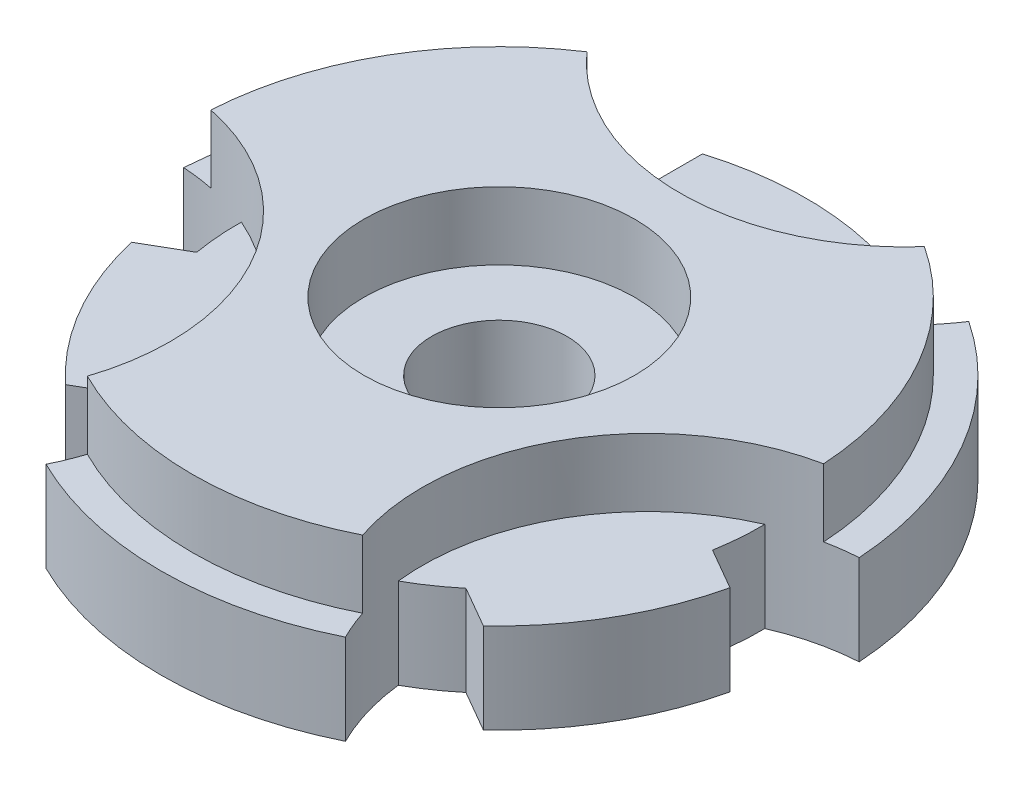
ISO-10303-21;
HEADER;
FILE_DESCRIPTION(('STEP AP214'),'2;1');
FILE_NAME('part.step','',(''),(''),'','','');
FILE_SCHEMA(('AUTOMOTIVE_DESIGN { 1 0 10303 214 1 1 1 1 }'));
ENDSEC;
DATA;
#1=APPLICATION_CONTEXT('core data for automotive mechanical design processes');
#2=APPLICATION_PROTOCOL_DEFINITION('international standard','automotive_design',2000,#1);
#3=PRODUCT_CONTEXT('',#1,'mechanical');
#4=PRODUCT('Part','Part','',(#3));
#5=PRODUCT_RELATED_PRODUCT_CATEGORY('part','',(#4));
#6=PRODUCT_DEFINITION_FORMATION('','',#4);
#7=PRODUCT_DEFINITION_CONTEXT('part definition',#1,'design');
#8=PRODUCT_DEFINITION('design','',#6,#7);
#9=PRODUCT_DEFINITION_SHAPE('','',#8);
#10=(LENGTH_UNIT() NAMED_UNIT(*) SI_UNIT(.MILLI.,.METRE.));
#11=(NAMED_UNIT(*) PLANE_ANGLE_UNIT() SI_UNIT($,.RADIAN.));
#12=(NAMED_UNIT(*) SI_UNIT($,.STERADIAN.) SOLID_ANGLE_UNIT());
#13=UNCERTAINTY_MEASURE_WITH_UNIT(LENGTH_MEASURE(1.E-05),#10,'distance_accuracy_value','');
#14=(GEOMETRIC_REPRESENTATION_CONTEXT(3) GLOBAL_UNCERTAINTY_ASSIGNED_CONTEXT((#13)) GLOBAL_UNIT_ASSIGNED_CONTEXT((#10,
#11,#12)) REPRESENTATION_CONTEXT('',''));
#15=CARTESIAN_POINT('',(0.,0.,0.));
#16=DIRECTION('',(0.,0.,1.));
#17=DIRECTION('',(1.,0.,0.));
#18=AXIS2_PLACEMENT_3D('',#15,#16,#17);
#19=CARTESIAN_POINT('',(0.,20.,0.));
#20=DIRECTION('',(0.,1.,0.));
#21=DIRECTION('',(0.,0.,1.));
#22=AXIS2_PLACEMENT_3D('',#19,#20,#21);
#23=PLANE('',#22);
#24=CARTESIAN_POINT('',(0.,20.,-90.));
#25=DIRECTION('',(0.,1.,0.));
#26=DIRECTION('',(0.,0.,1.));
#27=AXIS2_PLACEMENT_3D('',#24,#25,#26);
#28=CIRCLE('',#27,50.);
#29=CARTESIAN_POINT('',(29.7314648142334,20.,-49.8));
#30=VERTEX_POINT('',#29);
#31=CARTESIAN_POINT('',(-29.7314648142334,20.,-49.8));
#32=VERTEX_POINT('',#31);
#33=EDGE_CURVE('E11',#30,#32,#28,.F.);
#34=ORIENTED_EDGE('',*,*,#33,.F.);
#35=CARTESIAN_POINT('',(0.,20.,0.));
#36=DIRECTION('',(0.,1.,0.));
#37=DIRECTION('',(0.,0.,1.));
#38=AXIS2_PLACEMENT_3D('',#35,#36,#37);
#39=CIRCLE('',#38,58.);
#40=CARTESIAN_POINT('',(20.,20.,-54.4426303552648));
#41=VERTEX_POINT('',#40);
#42=EDGE_CURVE('E292',#30,#41,#39,.T.);
#43=ORIENTED_EDGE('',*,*,#42,.T.);
#44=DIRECTION('',(0.,0.,-1.));
#45=VECTOR('',#44,1.);
#46=CARTESIAN_POINT('',(20.,20.,0.));
#47=LINE('',#46,#45);
#48=CARTESIAN_POINT('',(20.,20.,-64.9923072370877));
#49=VERTEX_POINT('',#48);
#50=EDGE_CURVE('E291',#41,#49,#47,.T.);
#51=ORIENTED_EDGE('',*,*,#50,.T.);
#52=CARTESIAN_POINT('',(0.,20.,0.));
#53=DIRECTION('',(0.,1.,0.));
#54=DIRECTION('',(0.,0.,1.));
#55=AXIS2_PLACEMENT_3D('',#52,#53,#54);
#56=CIRCLE('',#55,68.);
#57=CARTESIAN_POINT('',(-20.,20.,-64.9923072370877));
#58=VERTEX_POINT('',#57);
#59=EDGE_CURVE('E293',#49,#58,#56,.T.);
#60=ORIENTED_EDGE('',*,*,#59,.T.);
#61=DIRECTION('',(0.,0.,-1.));
#62=VECTOR('',#61,1.);
#63=CARTESIAN_POINT('',(-20.,20.,0.));
#64=LINE('',#63,#62);
#65=CARTESIAN_POINT('',(-20.,20.,-54.4426303552648));
#66=VERTEX_POINT('',#65);
#67=EDGE_CURVE('E296',#66,#58,#64,.T.);
#68=ORIENTED_EDGE('',*,*,#67,.F.);
#69=CARTESIAN_POINT('',(0.,20.,0.));
#70=DIRECTION('',(0.,1.,0.));
#71=DIRECTION('',(0.,0.,1.));
#72=AXIS2_PLACEMENT_3D('',#69,#70,#71);
#73=CIRCLE('',#72,58.);
#74=EDGE_CURVE('E297',#66,#32,#73,.T.);
#75=ORIENTED_EDGE('',*,*,#74,.T.);
#76=EDGE_LOOP('',(#34,#43,#51,#60,#68,#75));
#77=FACE_BOUND('',#76,.T.);
#78=ADVANCED_FACE('F50',(#77),#23,.T.);
#79=CARTESIAN_POINT('',(0.,20.,0.));
#80=DIRECTION('',(0.,1.,0.));
#81=DIRECTION('',(0.,0.,1.));
#82=AXIS2_PLACEMENT_3D('',#79,#80,#81);
#83=CIRCLE('',#82,68.);
#84=CARTESIAN_POINT('',(67.8835572478328,20.,-3.97777015175732));
#85=VERTEX_POINT('',#84);
#86=CARTESIAN_POINT('',(37.3866286257533,20.,-56.8));
#87=VERTEX_POINT('',#86);
#88=EDGE_CURVE('E264',#85,#87,#83,.T.);
#89=ORIENTED_EDGE('',*,*,#88,.F.);
#90=CARTESIAN_POINT('',(77.9422863405995,20.,45.));
#91=DIRECTION('',(0.,1.,0.));
#92=DIRECTION('',(0.,0.,1.));
#93=AXIS2_PLACEMENT_3D('',#90,#91,#92);
#94=CIRCLE('',#93,50.0000000000004);
#95=CARTESIAN_POINT('',(74.8395240227173,20.,-4.90363579939614));
#96=VERTEX_POINT('',#95);
#97=EDGE_CURVE('E281',#96,#85,#94,.T.);
#98=ORIENTED_EDGE('',*,*,#97,.F.);
#99=CARTESIAN_POINT('',(0.,20.,0.));
#100=DIRECTION('',(0.,1.,0.));
#101=DIRECTION('',(0.,0.,1.));
#102=AXIS2_PLACEMENT_3D('',#99,#100,#101);
#103=CIRCLE('',#102,75.);
#104=CARTESIAN_POINT('',(41.6664351845422,20.,-62.3611111111112));
#105=VERTEX_POINT('',#104);
#106=EDGE_CURVE('E282',#96,#105,#103,.T.);
#107=ORIENTED_EDGE('',*,*,#106,.T.);
#108=CARTESIAN_POINT('',(0.,20.,-90.));
#109=DIRECTION('',(0.,1.,0.));
#110=DIRECTION('',(0.,0.,1.));
#111=AXIS2_PLACEMENT_3D('',#108,#109,#110);
#112=CIRCLE('',#111,50.);
#113=EDGE_CURVE('E287',#87,#105,#112,.T.);
#114=ORIENTED_EDGE('',*,*,#113,.F.);
#115=EDGE_LOOP('',(#89,#98,#107,#114));
#116=FACE_BOUND('',#115,.T.);
#117=ADVANCED_FACE('F531',(#116),#23,.T.);
#118=CARTESIAN_POINT('',(77.9422863405995,20.,45.));
#119=DIRECTION('',(0.,1.,0.));
#120=DIRECTION('',(0.,0.,1.));
#121=AXIS2_PLACEMENT_3D('',#118,#119,#120);
#122=CIRCLE('',#121,50.0000000000004);
#123=CARTESIAN_POINT('',(28.262332701348,20.,50.6482038208495));
#124=VERTEX_POINT('',#123);
#125=CARTESIAN_POINT('',(57.9937975155817,20.,-0.848203820849769));
#126=VERTEX_POINT('',#125);
#127=EDGE_CURVE('E57',#124,#126,#122,.F.);
#128=ORIENTED_EDGE('',*,*,#127,.F.);
#129=CARTESIAN_POINT('',(0.,20.,0.));
#130=DIRECTION('',(0.,1.,0.));
#131=DIRECTION('',(0.,0.,1.));
#132=AXIS2_PLACEMENT_3D('',#129,#130,#131);
#133=CIRCLE('',#132,58.);
#134=CARTESIAN_POINT('',(37.1487009365052,20.,44.5418232533212));
#135=VERTEX_POINT('',#134);
#136=EDGE_CURVE('E321',#124,#135,#133,.T.);
#137=ORIENTED_EDGE('',*,*,#136,.T.);
#138=DIRECTION('',(0.866025403784439,0.,0.5));
#139=VECTOR('',#138,1.);
#140=CARTESIAN_POINT('',(-10.,20.,17.3205080756888));
#141=LINE('',#140,#139);
#142=CARTESIAN_POINT('',(46.2849891178812,20.,49.8166616942326));
#143=VERTEX_POINT('',#142);
#144=EDGE_CURVE('E323',#135,#143,#141,.T.);
#145=ORIENTED_EDGE('',*,*,#144,.T.);
#146=CARTESIAN_POINT('',(0.,20.,0.));
#147=DIRECTION('',(0.,1.,0.));
#148=DIRECTION('',(0.,0.,1.));
#149=AXIS2_PLACEMENT_3D('',#146,#147,#148);
#150=CIRCLE('',#149,68.);
#151=CARTESIAN_POINT('',(66.2849891178812,20.,15.1756455428551));
#152=VERTEX_POINT('',#151);
#153=EDGE_CURVE('E324',#143,#152,#150,.T.);
#154=ORIENTED_EDGE('',*,*,#153,.T.);
#155=DIRECTION('',(0.866025403784439,0.,0.499999999999999));
#156=VECTOR('',#155,1.);
#157=CARTESIAN_POINT('',(9.99999999999997,20.,-17.3205080756888));
#158=LINE('',#157,#156);
#159=CARTESIAN_POINT('',(57.1487009365051,20.,9.90080710194361));
#160=VERTEX_POINT('',#159);
#161=EDGE_CURVE('E330',#160,#152,#158,.T.);
#162=ORIENTED_EDGE('',*,*,#161,.F.);
#163=CARTESIAN_POINT('',(0.,20.,0.));
#164=DIRECTION('',(0.,1.,0.));
#165=DIRECTION('',(0.,0.,1.));
#166=AXIS2_PLACEMENT_3D('',#163,#164,#165);
#167=CIRCLE('',#166,58.);
#168=EDGE_CURVE('E329',#160,#126,#167,.T.);
#169=ORIENTED_EDGE('',*,*,#168,.T.);
#170=EDGE_LOOP('',(#128,#137,#145,#154,#162,#169));
#171=FACE_BOUND('',#170,.T.);
#172=ADVANCED_FACE('F541',(#171),#23,.T.);
#173=CARTESIAN_POINT('',(0.,20.,0.));
#174=DIRECTION('',(0.,1.,0.));
#175=DIRECTION('',(0.,0.,1.));
#176=AXIS2_PLACEMENT_3D('',#173,#174,#175);
#177=CIRCLE('',#176,68.);
#178=CARTESIAN_POINT('',(-30.4969286220787,20.,60.7777701517573));
#179=VERTEX_POINT('',#178);
#180=CARTESIAN_POINT('',(30.4969286220791,20.,60.7777701517571));
#181=VERTEX_POINT('',#180);
#182=EDGE_CURVE('E66',#179,#181,#177,.T.);
#183=ORIENTED_EDGE('',*,*,#182,.F.);
#184=CARTESIAN_POINT('',(-77.9422863405995,20.,45.));
#185=DIRECTION('',(0.,1.,0.));
#186=DIRECTION('',(0.,0.,1.));
#187=AXIS2_PLACEMENT_3D('',#184,#185,#186);
#188=CIRCLE('',#187,50.0000000000008);
#189=CARTESIAN_POINT('',(-33.1730888381744,20.,67.2647469105072));
#190=VERTEX_POINT('',#189);
#191=EDGE_CURVE('E306',#190,#179,#188,.T.);
#192=ORIENTED_EDGE('',*,*,#191,.F.);
#193=CARTESIAN_POINT('',(0.,20.,0.));
#194=DIRECTION('',(0.,1.,0.));
#195=DIRECTION('',(0.,0.,1.));
#196=AXIS2_PLACEMENT_3D('',#193,#194,#195);
#197=CIRCLE('',#196,75.);
#198=CARTESIAN_POINT('',(33.1730888381748,20.,67.264746910507));
#199=VERTEX_POINT('',#198);
#200=EDGE_CURVE('E317',#190,#199,#197,.T.);
#201=ORIENTED_EDGE('',*,*,#200,.T.);
#202=EDGE_CURVE('E63',#181,#199,#94,.T.);
#203=ORIENTED_EDGE('',*,*,#202,.F.);
#204=EDGE_LOOP('',(#183,#192,#201,#203));
#205=FACE_BOUND('',#204,.T.);
#206=ADVANCED_FACE('F473',(#205),#23,.T.);
#207=CARTESIAN_POINT('',(-77.9422863405995,20.,45.));
#208=DIRECTION('',(0.,1.,0.));
#209=DIRECTION('',(0.,0.,1.));
#210=AXIS2_PLACEMENT_3D('',#207,#208,#209);
#211=CIRCLE('',#210,50.0000000000008);
#212=CARTESIAN_POINT('',(-57.9937975155817,20.,-0.848203820850199));
#213=VERTEX_POINT('',#212);
#214=CARTESIAN_POINT('',(-28.2623327013475,20.,50.6482038208498));
#215=VERTEX_POINT('',#214);
#216=EDGE_CURVE('E437',#213,#215,#211,.F.);
#217=ORIENTED_EDGE('',*,*,#216,.F.);
#218=CARTESIAN_POINT('',(0.,20.,0.));
#219=DIRECTION('',(0.,1.,0.));
#220=DIRECTION('',(0.,0.,1.));
#221=AXIS2_PLACEMENT_3D('',#218,#219,#220);
#222=CIRCLE('',#221,58.);
#223=CARTESIAN_POINT('',(-57.1487009365051,20.,9.90080710194364));
#224=VERTEX_POINT('',#223);
#225=EDGE_CURVE('E307',#213,#224,#222,.T.);
#226=ORIENTED_EDGE('',*,*,#225,.T.);
#227=DIRECTION('',(-0.866025403784439,0.,0.5));
#228=VECTOR('',#227,1.);
#229=CARTESIAN_POINT('',(-9.99999999999997,20.,-17.3205080756887));
#230=LINE('',#229,#228);
#231=CARTESIAN_POINT('',(-66.2849891178812,20.,15.1756455428551));
#232=VERTEX_POINT('',#231);
#233=EDGE_CURVE('E309',#224,#232,#230,.T.);
#234=ORIENTED_EDGE('',*,*,#233,.T.);
#235=CARTESIAN_POINT('',(0.,20.,0.));
#236=DIRECTION('',(0.,1.,0.));
#237=DIRECTION('',(0.,0.,1.));
#238=AXIS2_PLACEMENT_3D('',#235,#236,#237);
#239=CIRCLE('',#238,68.);
#240=CARTESIAN_POINT('',(-46.2849891178811,20.,49.8166616942326));
#241=VERTEX_POINT('',#240);
#242=EDGE_CURVE('E315',#232,#241,#239,.T.);
#243=ORIENTED_EDGE('',*,*,#242,.T.);
#244=DIRECTION('',(-0.866025403784439,0.,0.5));
#245=VECTOR('',#244,1.);
#246=CARTESIAN_POINT('',(10.,20.,17.3205080756888));
#247=LINE('',#246,#245);
#248=CARTESIAN_POINT('',(-37.1487009365051,20.,44.5418232533212));
#249=VERTEX_POINT('',#248);
#250=EDGE_CURVE('E314',#249,#241,#247,.T.);
#251=ORIENTED_EDGE('',*,*,#250,.F.);
#252=CARTESIAN_POINT('',(0.,20.,0.));
#253=DIRECTION('',(0.,1.,0.));
#254=DIRECTION('',(0.,0.,1.));
#255=AXIS2_PLACEMENT_3D('',#252,#253,#254);
#256=CIRCLE('',#255,58.);
#257=EDGE_CURVE('E320',#249,#215,#256,.T.);
#258=ORIENTED_EDGE('',*,*,#257,.T.);
#259=EDGE_LOOP('',(#217,#226,#234,#243,#251,#258));
#260=FACE_BOUND('',#259,.T.);
#261=ADVANCED_FACE('F547',(#260),#23,.T.);
#262=CARTESIAN_POINT('',(0.,20.,0.));
#263=DIRECTION('',(0.,-1.,0.));
#264=DIRECTION('',(0.,0.,-1.));
#265=AXIS2_PLACEMENT_3D('',#262,#263,#264);
#266=CYLINDRICAL_SURFACE('',#265,75.);
#267=CARTESIAN_POINT('',(0.,0.,0.));
#268=DIRECTION('',(0.,1.,0.));
#269=DIRECTION('',(0.,0.,1.));
#270=AXIS2_PLACEMENT_3D('',#267,#268,#269);
#271=CIRCLE('',#270,75.);
#272=CARTESIAN_POINT('',(74.8395240227173,0.,-4.90363579939614));
#273=VERTEX_POINT('',#272);
#274=CARTESIAN_POINT('',(41.6664351845422,0.,-62.3611111111112));
#275=VERTEX_POINT('',#274);
#276=EDGE_CURVE('E274',#273,#275,#271,.T.);
#277=ORIENTED_EDGE('',*,*,#276,.T.);
#278=DIRECTION('',(0.,-1.,0.));
#279=VECTOR('',#278,1.);
#280=CARTESIAN_POINT('',(41.6664351845422,20.,-62.3611111111112));
#281=LINE('',#280,#279);
#282=EDGE_CURVE('E434',#105,#275,#281,.T.);
#283=ORIENTED_EDGE('',*,*,#282,.F.);
#284=ORIENTED_EDGE('',*,*,#106,.F.);
#285=DIRECTION('',(0.,-1.,0.));
#286=VECTOR('',#285,1.);
#287=CARTESIAN_POINT('',(74.8395240227173,20.,-4.90363579939614));
#288=LINE('',#287,#286);
#289=EDGE_CURVE('E51',#96,#273,#288,.T.);
#290=ORIENTED_EDGE('',*,*,#289,.T.);
#291=EDGE_LOOP('',(#277,#283,#284,#290));
#292=FACE_BOUND('',#291,.T.);
#293=ADVANCED_FACE('F47',(#292),#266,.T.);
#294=CARTESIAN_POINT('',(0.,20.,0.));
#295=DIRECTION('',(0.,-1.,0.));
#296=DIRECTION('',(0.,0.,-1.));
#297=AXIS2_PLACEMENT_3D('',#294,#295,#296);
#298=CYLINDRICAL_SURFACE('',#297,58.);
#299=CARTESIAN_POINT('',(0.,0.,0.));
#300=DIRECTION('',(0.,1.,0.));
#301=DIRECTION('',(0.,0.,1.));
#302=AXIS2_PLACEMENT_3D('',#299,#300,#301);
#303=CIRCLE('',#302,58.);
#304=CARTESIAN_POINT('',(29.7314648142334,0.,-49.8));
#305=VERTEX_POINT('',#304);
#306=CARTESIAN_POINT('',(20.,0.,-54.4426303552648));
#307=VERTEX_POINT('',#306);
#308=EDGE_CURVE('E340',#305,#307,#303,.T.);
#309=ORIENTED_EDGE('',*,*,#308,.T.);
#310=DIRECTION('',(0.,-1.,0.));
#311=VECTOR('',#310,1.);
#312=CARTESIAN_POINT('',(20.,20.,-54.4426303552648));
#313=LINE('',#312,#311);
#314=EDGE_CURVE('E431',#41,#307,#313,.T.);
#315=ORIENTED_EDGE('',*,*,#314,.F.);
#316=ORIENTED_EDGE('',*,*,#42,.F.);
#317=DIRECTION('',(0.,-1.,0.));
#318=VECTOR('',#317,1.);
#319=CARTESIAN_POINT('',(29.7314648142334,20.,-49.8));
#320=LINE('',#319,#318);
#321=EDGE_CURVE('E432',#30,#305,#320,.T.);
#322=ORIENTED_EDGE('',*,*,#321,.T.);
#323=EDGE_LOOP('',(#309,#315,#316,#322));
#324=FACE_BOUND('',#323,.T.);
#325=ADVANCED_FACE('F562',(#324),#298,.T.);
#326=CARTESIAN_POINT('',(20.,20.,0.));
#327=DIRECTION('',(-1.,0.,0.));
#328=DIRECTION('',(0.,0.,1.));
#329=AXIS2_PLACEMENT_3D('',#326,#327,#328);
#330=PLANE('',#329);
#331=DIRECTION('',(0.,0.,-1.));
#332=VECTOR('',#331,1.);
#333=CARTESIAN_POINT('',(20.,0.,0.));
#334=LINE('',#333,#332);
#335=CARTESIAN_POINT('',(20.,0.,-64.9923072370877));
#336=VERTEX_POINT('',#335);
#337=EDGE_CURVE('E343',#307,#336,#334,.T.);
#338=ORIENTED_EDGE('',*,*,#337,.T.);
#339=DIRECTION('',(0.,-1.,0.));
#340=VECTOR('',#339,1.);
#341=CARTESIAN_POINT('',(20.,20.,-64.9923072370877));
#342=LINE('',#341,#340);
#343=EDGE_CURVE('E428',#49,#336,#342,.T.);
#344=ORIENTED_EDGE('',*,*,#343,.F.);
#345=ORIENTED_EDGE('',*,*,#50,.F.);
#346=ORIENTED_EDGE('',*,*,#314,.T.);
#347=EDGE_LOOP('',(#338,#344,#345,#346));
#348=FACE_BOUND('',#347,.T.);
#349=ADVANCED_FACE('F653',(#348),#330,.F.);
#350=CARTESIAN_POINT('',(0.,20.,0.));
#351=DIRECTION('',(0.,-1.,0.));
#352=DIRECTION('',(0.,0.,-1.));
#353=AXIS2_PLACEMENT_3D('',#350,#351,#352);
#354=CYLINDRICAL_SURFACE('',#353,68.);
#355=CARTESIAN_POINT('',(0.,0.,0.));
#356=DIRECTION('',(0.,1.,0.));
#357=DIRECTION('',(0.,0.,1.));
#358=AXIS2_PLACEMENT_3D('',#355,#356,#357);
#359=CIRCLE('',#358,68.);
#360=CARTESIAN_POINT('',(-20.,0.,-64.9923072370877));
#361=VERTEX_POINT('',#360);
#362=EDGE_CURVE('E341',#336,#361,#359,.T.);
#363=ORIENTED_EDGE('',*,*,#362,.T.);
#364=DIRECTION('',(0.,-1.,0.));
#365=VECTOR('',#364,1.);
#366=CARTESIAN_POINT('',(-20.,20.,-64.9923072370877));
#367=LINE('',#366,#365);
#368=EDGE_CURVE('E426',#58,#361,#367,.T.);
#369=ORIENTED_EDGE('',*,*,#368,.F.);
#370=ORIENTED_EDGE('',*,*,#59,.F.);
#371=ORIENTED_EDGE('',*,*,#343,.T.);
#372=EDGE_LOOP('',(#363,#369,#370,#371));
#373=FACE_BOUND('',#372,.T.);
#374=ADVANCED_FACE('F647',(#373),#354,.T.);
#375=CARTESIAN_POINT('',(-20.,20.,0.));
#376=DIRECTION('',(-1.,0.,0.));
#377=DIRECTION('',(0.,0.,1.));
#378=AXIS2_PLACEMENT_3D('',#375,#376,#377);
#379=PLANE('',#378);
#380=DIRECTION('',(0.,0.,-1.));
#381=VECTOR('',#380,1.);
#382=CARTESIAN_POINT('',(-20.,0.,0.));
#383=LINE('',#382,#381);
#384=CARTESIAN_POINT('',(-20.,0.,-54.4426303552648));
#385=VERTEX_POINT('',#384);
#386=EDGE_CURVE('E347',#385,#361,#383,.T.);
#387=ORIENTED_EDGE('',*,*,#386,.F.);
#388=DIRECTION('',(0.,-1.,0.));
#389=VECTOR('',#388,1.);
#390=CARTESIAN_POINT('',(-20.,20.,-54.4426303552648));
#391=LINE('',#390,#389);
#392=EDGE_CURVE('E424',#66,#385,#391,.T.);
#393=ORIENTED_EDGE('',*,*,#392,.F.);
#394=ORIENTED_EDGE('',*,*,#67,.T.);
#395=ORIENTED_EDGE('',*,*,#368,.T.);
#396=EDGE_LOOP('',(#387,#393,#394,#395));
#397=FACE_BOUND('',#396,.T.);
#398=ADVANCED_FACE('F650',(#397),#379,.T.);
#399=CARTESIAN_POINT('',(0.,20.,0.));
#400=DIRECTION('',(0.,-1.,0.));
#401=DIRECTION('',(0.,0.,-1.));
#402=AXIS2_PLACEMENT_3D('',#399,#400,#401);
#403=CYLINDRICAL_SURFACE('',#402,58.);
#404=CARTESIAN_POINT('',(0.,0.,0.));
#405=DIRECTION('',(0.,1.,0.));
#406=DIRECTION('',(0.,0.,1.));
#407=AXIS2_PLACEMENT_3D('',#404,#405,#406);
#408=CIRCLE('',#407,58.);
#409=CARTESIAN_POINT('',(-29.7314648142334,0.,-49.8));
#410=VERTEX_POINT('',#409);
#411=EDGE_CURVE('E349',#385,#410,#408,.T.);
#412=ORIENTED_EDGE('',*,*,#411,.T.);
#413=DIRECTION('',(0.,-1.,0.));
#414=VECTOR('',#413,1.);
#415=CARTESIAN_POINT('',(-29.7314648142334,20.,-49.8));
#416=LINE('',#415,#414);
#417=EDGE_CURVE('E425',#32,#410,#416,.T.);
#418=ORIENTED_EDGE('',*,*,#417,.F.);
#419=ORIENTED_EDGE('',*,*,#74,.F.);
#420=ORIENTED_EDGE('',*,*,#392,.T.);
#421=EDGE_LOOP('',(#412,#418,#419,#420));
#422=FACE_BOUND('',#421,.T.);
#423=ADVANCED_FACE('F624',(#422),#403,.T.);
#424=CARTESIAN_POINT('',(0.,20.,-90.));
#425=DIRECTION('',(0.,-1.,0.));
#426=DIRECTION('',(0.,0.,-1.));
#427=AXIS2_PLACEMENT_3D('',#424,#425,#426);
#428=CYLINDRICAL_SURFACE('',#427,50.);
#429=CARTESIAN_POINT('',(0.,0.,-90.));
#430=DIRECTION('',(0.,1.,0.));
#431=DIRECTION('',(0.,0.,1.));
#432=AXIS2_PLACEMENT_3D('',#429,#430,#431);
#433=CIRCLE('',#432,50.);
#434=CARTESIAN_POINT('',(-41.6664351845421,0.,-62.3611111111111));
#435=VERTEX_POINT('',#434);
#436=EDGE_CURVE('E338',#435,#410,#433,.T.);
#437=ORIENTED_EDGE('',*,*,#436,.F.);
#438=DIRECTION('',(0.,-1.,0.));
#439=VECTOR('',#438,1.);
#440=CARTESIAN_POINT('',(-41.6664351845421,20.,-62.3611111111111));
#441=LINE('',#440,#439);
#442=CARTESIAN_POINT('',(-41.6664351845421,20.,-62.3611111111111));
#443=VERTEX_POINT('',#442);
#444=EDGE_CURVE('E419',#443,#435,#441,.T.);
#445=ORIENTED_EDGE('',*,*,#444,.F.);
#446=CARTESIAN_POINT('',(-37.3866286257533,20.,-56.8));
#447=VERTEX_POINT('',#446);
#448=EDGE_CURVE('E271',#443,#447,#112,.T.);
#449=ORIENTED_EDGE('',*,*,#448,.T.);
#450=DIRECTION('',(0.,-1.,0.));
#451=VECTOR('',#450,1.);
#452=CARTESIAN_POINT('',(-37.3866286257533,35.,-56.8));
#453=LINE('',#452,#451);
#454=CARTESIAN_POINT('',(-37.3866286257533,35.,-56.8));
#455=VERTEX_POINT('',#454);
#456=EDGE_CURVE('E249',#455,#447,#453,.T.);
#457=ORIENTED_EDGE('',*,*,#456,.F.);
#458=CARTESIAN_POINT('',(0.,35.,-90.));
#459=DIRECTION('',(0.,1.,0.));
#460=DIRECTION('',(0.,0.,1.));
#461=AXIS2_PLACEMENT_3D('',#458,#459,#460);
#462=CIRCLE('',#461,50.);
#463=CARTESIAN_POINT('',(37.3866286257533,35.,-56.8));
#464=VERTEX_POINT('',#463);
#465=EDGE_CURVE('E258',#464,#455,#462,.F.);
#466=ORIENTED_EDGE('',*,*,#465,.F.);
#467=DIRECTION('',(0.,-1.,0.));
#468=VECTOR('',#467,1.);
#469=CARTESIAN_POINT('',(37.3866286257533,35.,-56.8));
#470=LINE('',#469,#468);
#471=EDGE_CURVE('E452',#464,#87,#470,.T.);
#472=ORIENTED_EDGE('',*,*,#471,.T.);
#473=ORIENTED_EDGE('',*,*,#113,.T.);
#474=ORIENTED_EDGE('',*,*,#282,.T.);
#475=EDGE_CURVE('E333',#305,#275,#433,.T.);
#476=ORIENTED_EDGE('',*,*,#475,.F.);
#477=ORIENTED_EDGE('',*,*,#321,.F.);
#478=ORIENTED_EDGE('',*,*,#33,.T.);
#479=ORIENTED_EDGE('',*,*,#417,.T.);
#480=EDGE_LOOP('',(#437,#445,#449,#457,#466,#472,#473,#474,#476,#477,#478,#479));
#481=FACE_BOUND('',#480,.T.);
#482=ADVANCED_FACE('F267',(#481),#428,.F.);
#483=CARTESIAN_POINT('',(0.,20.,0.));
#484=DIRECTION('',(0.,-1.,0.));
#485=DIRECTION('',(0.,0.,-1.));
#486=AXIS2_PLACEMENT_3D('',#483,#484,#485);
#487=CYLINDRICAL_SURFACE('',#486,75.);
#488=CARTESIAN_POINT('',(0.,0.,0.));
#489=DIRECTION('',(0.,1.,0.));
#490=DIRECTION('',(0.,0.,1.));
#491=AXIS2_PLACEMENT_3D('',#488,#489,#490);
#492=CIRCLE('',#491,75.);
#493=CARTESIAN_POINT('',(-74.8395240227173,0.,-4.90363579939651));
#494=VERTEX_POINT('',#493);
#495=EDGE_CURVE('E351',#435,#494,#492,.T.);
#496=ORIENTED_EDGE('',*,*,#495,.T.);
#497=DIRECTION('',(0.,-1.,0.));
#498=VECTOR('',#497,1.);
#499=CARTESIAN_POINT('',(-74.8395240227173,20.,-4.90363579939651));
#500=LINE('',#499,#498);
#501=CARTESIAN_POINT('',(-74.8395240227173,20.,-4.90363579939651));
#502=VERTEX_POINT('',#501);
#503=EDGE_CURVE('E416',#502,#494,#500,.T.);
#504=ORIENTED_EDGE('',*,*,#503,.F.);
#505=CARTESIAN_POINT('',(0.,20.,0.));
#506=DIRECTION('',(0.,1.,0.));
#507=DIRECTION('',(0.,0.,1.));
#508=AXIS2_PLACEMENT_3D('',#505,#506,#507);
#509=CIRCLE('',#508,75.);
#510=EDGE_CURVE('E305',#443,#502,#509,.T.);
#511=ORIENTED_EDGE('',*,*,#510,.F.);
#512=ORIENTED_EDGE('',*,*,#444,.T.);
#513=EDGE_LOOP('',(#496,#504,#511,#512));
#514=FACE_BOUND('',#513,.T.);
#515=ADVANCED_FACE('F635',(#514),#487,.T.);
#516=CARTESIAN_POINT('',(0.,20.,0.));
#517=DIRECTION('',(0.,-1.,0.));
#518=DIRECTION('',(0.,0.,-1.));
#519=AXIS2_PLACEMENT_3D('',#516,#517,#518);
#520=CYLINDRICAL_SURFACE('',#519,58.);
#521=CARTESIAN_POINT('',(0.,0.,0.));
#522=DIRECTION('',(0.,1.,0.));
#523=DIRECTION('',(0.,0.,1.));
#524=AXIS2_PLACEMENT_3D('',#521,#522,#523);
#525=CIRCLE('',#524,58.);
#526=CARTESIAN_POINT('',(-57.9937975155817,0.,-0.848203820850199));
#527=VERTEX_POINT('',#526);
#528=CARTESIAN_POINT('',(-57.1487009365051,0.,9.90080710194364));
#529=VERTEX_POINT('',#528);
#530=EDGE_CURVE('E356',#527,#529,#525,.T.);
#531=ORIENTED_EDGE('',*,*,#530,.T.);
#532=DIRECTION('',(0.,-1.,0.));
#533=VECTOR('',#532,1.);
#534=CARTESIAN_POINT('',(-57.1487009365051,20.,9.90080710194364));
#535=LINE('',#534,#533);
#536=EDGE_CURVE('E411',#224,#529,#535,.T.);
#537=ORIENTED_EDGE('',*,*,#536,.F.);
#538=ORIENTED_EDGE('',*,*,#225,.F.);
#539=DIRECTION('',(0.,-1.,0.));
#540=VECTOR('',#539,1.);
#541=CARTESIAN_POINT('',(-57.9937975155817,20.,-0.848203820850199));
#542=LINE('',#541,#540);
#543=EDGE_CURVE('E418',#213,#527,#542,.T.);
#544=ORIENTED_EDGE('',*,*,#543,.T.);
#545=EDGE_LOOP('',(#531,#537,#538,#544));
#546=FACE_BOUND('',#545,.T.);
#547=ADVANCED_FACE('F575',(#546),#520,.T.);
#548=CARTESIAN_POINT('',(-9.99999999999997,20.,-17.3205080756887));
#549=DIRECTION('',(0.5,0.,0.866025403784439));
#550=DIRECTION('',(0.866025403784439,0.,-0.5));
#551=AXIS2_PLACEMENT_3D('',#548,#549,#550);
#552=PLANE('',#551);
#553=DIRECTION('',(-0.866025403784439,0.,0.5));
#554=VECTOR('',#553,1.);
#555=CARTESIAN_POINT('',(-9.99999999999997,0.,-17.3205080756887));
#556=LINE('',#555,#554);
#557=CARTESIAN_POINT('',(-66.2849891178812,0.,15.1756455428551));
#558=VERTEX_POINT('',#557);
#559=EDGE_CURVE('E363',#529,#558,#556,.T.);
#560=ORIENTED_EDGE('',*,*,#559,.T.);
#561=DIRECTION('',(0.,-1.,0.));
#562=VECTOR('',#561,1.);
#563=CARTESIAN_POINT('',(-66.2849891178812,20.,15.1756455428551));
#564=LINE('',#563,#562);
#565=EDGE_CURVE('E407',#232,#558,#564,.T.);
#566=ORIENTED_EDGE('',*,*,#565,.F.);
#567=ORIENTED_EDGE('',*,*,#233,.F.);
#568=ORIENTED_EDGE('',*,*,#536,.T.);
#569=EDGE_LOOP('',(#560,#566,#567,#568));
#570=FACE_BOUND('',#569,.T.);
#571=ADVANCED_FACE('F576',(#570),#552,.F.);
#572=CARTESIAN_POINT('',(0.,20.,0.));
#573=DIRECTION('',(0.,-1.,0.));
#574=DIRECTION('',(0.,0.,-1.));
#575=AXIS2_PLACEMENT_3D('',#572,#573,#574);
#576=CYLINDRICAL_SURFACE('',#575,68.);
#577=CARTESIAN_POINT('',(0.,0.,0.));
#578=DIRECTION('',(0.,1.,0.));
#579=DIRECTION('',(0.,0.,1.));
#580=AXIS2_PLACEMENT_3D('',#577,#578,#579);
#581=CIRCLE('',#580,68.);
#582=CARTESIAN_POINT('',(-46.2849891178811,0.,49.8166616942326));
#583=VERTEX_POINT('',#582);
#584=EDGE_CURVE('E361',#558,#583,#581,.T.);
#585=ORIENTED_EDGE('',*,*,#584,.T.);
#586=DIRECTION('',(0.,-1.,0.));
#587=VECTOR('',#586,1.);
#588=CARTESIAN_POINT('',(-46.2849891178811,20.,49.8166616942326));
#589=LINE('',#588,#587);
#590=EDGE_CURVE('E410',#241,#583,#589,.T.);
#591=ORIENTED_EDGE('',*,*,#590,.F.);
#592=ORIENTED_EDGE('',*,*,#242,.F.);
#593=ORIENTED_EDGE('',*,*,#565,.T.);
#594=EDGE_LOOP('',(#585,#591,#592,#593));
#595=FACE_BOUND('',#594,.T.);
#596=ADVANCED_FACE('F582',(#595),#576,.T.);
#597=CARTESIAN_POINT('',(10.,20.,17.3205080756888));
#598=DIRECTION('',(0.5,0.,0.866025403784439));
#599=DIRECTION('',(0.866025403784439,0.,-0.5));
#600=AXIS2_PLACEMENT_3D('',#597,#598,#599);
#601=PLANE('',#600);
#602=DIRECTION('',(-0.866025403784439,0.,0.5));
#603=VECTOR('',#602,1.);
#604=CARTESIAN_POINT('',(10.,0.,17.3205080756888));
#605=LINE('',#604,#603);
#606=CARTESIAN_POINT('',(-37.1487009365051,0.,44.5418232533212));
#607=VERTEX_POINT('',#606);
#608=EDGE_CURVE('E368',#607,#583,#605,.T.);
#609=ORIENTED_EDGE('',*,*,#608,.F.);
#610=DIRECTION('',(0.,-1.,0.));
#611=VECTOR('',#610,1.);
#612=CARTESIAN_POINT('',(-37.1487009365051,20.,44.5418232533212));
#613=LINE('',#612,#611);
#614=EDGE_CURVE('E409',#249,#607,#613,.T.);
#615=ORIENTED_EDGE('',*,*,#614,.F.);
#616=ORIENTED_EDGE('',*,*,#250,.T.);
#617=ORIENTED_EDGE('',*,*,#590,.T.);
#618=EDGE_LOOP('',(#609,#615,#616,#617));
#619=FACE_BOUND('',#618,.T.);
#620=ADVANCED_FACE('F588',(#619),#601,.T.);
#621=CARTESIAN_POINT('',(0.,20.,0.));
#622=DIRECTION('',(0.,-1.,0.));
#623=DIRECTION('',(0.,0.,-1.));
#624=AXIS2_PLACEMENT_3D('',#621,#622,#623);
#625=CYLINDRICAL_SURFACE('',#624,58.);
#626=CARTESIAN_POINT('',(0.,0.,0.));
#627=DIRECTION('',(0.,1.,0.));
#628=DIRECTION('',(0.,0.,1.));
#629=AXIS2_PLACEMENT_3D('',#626,#627,#628);
#630=CIRCLE('',#629,58.);
#631=CARTESIAN_POINT('',(-28.2623327013475,0.,50.6482038208498));
#632=VERTEX_POINT('',#631);
#633=EDGE_CURVE('E369',#607,#632,#630,.T.);
#634=ORIENTED_EDGE('',*,*,#633,.T.);
#635=DIRECTION('',(0.,-1.,0.));
#636=VECTOR('',#635,1.);
#637=CARTESIAN_POINT('',(-28.2623327013475,20.,50.6482038208498));
#638=LINE('',#637,#636);
#639=EDGE_CURVE('E404',#215,#632,#638,.T.);
#640=ORIENTED_EDGE('',*,*,#639,.F.);
#641=ORIENTED_EDGE('',*,*,#257,.F.);
#642=ORIENTED_EDGE('',*,*,#614,.T.);
#643=EDGE_LOOP('',(#634,#640,#641,#642));
#644=FACE_BOUND('',#643,.T.);
#645=ADVANCED_FACE('F589',(#644),#625,.T.);
#646=CARTESIAN_POINT('',(-77.9422863405995,20.,45.));
#647=DIRECTION('',(0.,-1.,0.));
#648=DIRECTION('',(0.,0.,-1.));
#649=AXIS2_PLACEMENT_3D('',#646,#647,#648);
#650=CYLINDRICAL_SURFACE('',#649,50.0000000000008);
#651=CARTESIAN_POINT('',(-77.9422863405995,0.,45.));
#652=DIRECTION('',(0.,1.,0.));
#653=DIRECTION('',(0.,0.,1.));
#654=AXIS2_PLACEMENT_3D('',#651,#652,#653);
#655=CIRCLE('',#654,50.0000000000008);
#656=CARTESIAN_POINT('',(-33.1730888381744,0.,67.2647469105072));
#657=VERTEX_POINT('',#656);
#658=EDGE_CURVE('E357',#657,#632,#655,.T.);
#659=ORIENTED_EDGE('',*,*,#658,.F.);
#660=DIRECTION('',(0.,-1.,0.));
#661=VECTOR('',#660,1.);
#662=CARTESIAN_POINT('',(-33.1730888381744,20.,67.2647469105072));
#663=LINE('',#662,#661);
#664=EDGE_CURVE('E405',#190,#657,#663,.T.);
#665=ORIENTED_EDGE('',*,*,#664,.F.);
#666=ORIENTED_EDGE('',*,*,#191,.T.);
#667=DIRECTION('',(0.,-1.,0.));
#668=VECTOR('',#667,1.);
#669=CARTESIAN_POINT('',(-30.4969286220787,35.,60.7777701517573));
#670=LINE('',#669,#668);
#671=CARTESIAN_POINT('',(-30.4969286220787,35.,60.7777701517573));
#672=VERTEX_POINT('',#671);
#673=EDGE_CURVE('E279',#672,#179,#670,.T.);
#674=ORIENTED_EDGE('',*,*,#673,.F.);
#675=CARTESIAN_POINT('',(-77.9422863405995,35.,45.));
#676=DIRECTION('',(0.,1.,0.));
#677=DIRECTION('',(0.,0.,1.));
#678=AXIS2_PLACEMENT_3D('',#675,#676,#677);
#679=CIRCLE('',#678,50.0000000000008);
#680=CARTESIAN_POINT('',(-67.8835572478328,35.,-3.97777015175771));
#681=VERTEX_POINT('',#680);
#682=EDGE_CURVE('E254',#681,#672,#679,.F.);
#683=ORIENTED_EDGE('',*,*,#682,.F.);
#684=DIRECTION('',(0.,-1.,0.));
#685=VECTOR('',#684,1.);
#686=CARTESIAN_POINT('',(-67.8835572478328,35.,-3.97777015175771));
#687=LINE('',#686,#685);
#688=CARTESIAN_POINT('',(-67.8835572478328,20.,-3.97777015175771));
#689=VERTEX_POINT('',#688);
#690=EDGE_CURVE('E252',#681,#689,#687,.T.);
#691=ORIENTED_EDGE('',*,*,#690,.T.);
#692=EDGE_CURVE('E304',#689,#502,#188,.T.);
#693=ORIENTED_EDGE('',*,*,#692,.T.);
#694=ORIENTED_EDGE('',*,*,#503,.T.);
#695=EDGE_CURVE('E352',#527,#494,#655,.T.);
#696=ORIENTED_EDGE('',*,*,#695,.F.);
#697=ORIENTED_EDGE('',*,*,#543,.F.);
#698=ORIENTED_EDGE('',*,*,#216,.T.);
#699=ORIENTED_EDGE('',*,*,#639,.T.);
#700=EDGE_LOOP('',(#659,#665,#666,#674,#683,#691,#693,#694,#696,#697,#698,#699));
#701=FACE_BOUND('',#700,.T.);
#702=ADVANCED_FACE('F467',(#701),#650,.F.);
#703=CARTESIAN_POINT('',(0.,20.,0.));
#704=DIRECTION('',(0.,-1.,0.));
#705=DIRECTION('',(0.,0.,-1.));
#706=AXIS2_PLACEMENT_3D('',#703,#704,#705);
#707=CYLINDRICAL_SURFACE('',#706,75.);
#708=CARTESIAN_POINT('',(0.,0.,0.));
#709=DIRECTION('',(0.,1.,0.));
#710=DIRECTION('',(0.,0.,1.));
#711=AXIS2_PLACEMENT_3D('',#708,#709,#710);
#712=CIRCLE('',#711,75.);
#713=CARTESIAN_POINT('',(33.1730888381748,0.,67.264746910507));
#714=VERTEX_POINT('',#713);
#715=EDGE_CURVE('E375',#657,#714,#712,.T.);
#716=ORIENTED_EDGE('',*,*,#715,.T.);
#717=DIRECTION('',(0.,-1.,0.));
#718=VECTOR('',#717,1.);
#719=CARTESIAN_POINT('',(33.1730888381748,20.,67.264746910507));
#720=LINE('',#719,#718);
#721=EDGE_CURVE('E399',#199,#714,#720,.T.);
#722=ORIENTED_EDGE('',*,*,#721,.F.);
#723=ORIENTED_EDGE('',*,*,#200,.F.);
#724=ORIENTED_EDGE('',*,*,#664,.T.);
#725=EDGE_LOOP('',(#716,#722,#723,#724));
#726=FACE_BOUND('',#725,.T.);
#727=ADVANCED_FACE('F475',(#726),#707,.T.);
#728=CARTESIAN_POINT('',(77.9422863405995,20.,45.));
#729=DIRECTION('',(0.,-1.,0.));
#730=DIRECTION('',(0.,0.,-1.));
#731=AXIS2_PLACEMENT_3D('',#728,#729,#730);
#732=CYLINDRICAL_SURFACE('',#731,50.0000000000004);
#733=CARTESIAN_POINT('',(77.9422863405995,0.,45.));
#734=DIRECTION('',(0.,1.,0.));
#735=DIRECTION('',(0.,0.,1.));
#736=AXIS2_PLACEMENT_3D('',#733,#734,#735);
#737=CIRCLE('',#736,50.0000000000004);
#738=CARTESIAN_POINT('',(28.262332701348,0.,50.6482038208495));
#739=VERTEX_POINT('',#738);
#740=EDGE_CURVE('E280',#739,#714,#737,.T.);
#741=ORIENTED_EDGE('',*,*,#740,.F.);
#742=DIRECTION('',(0.,-1.,0.));
#743=VECTOR('',#742,1.);
#744=CARTESIAN_POINT('',(28.262332701348,20.,50.6482038208495));
#745=LINE('',#744,#743);
#746=EDGE_CURVE('E396',#124,#739,#745,.T.);
#747=ORIENTED_EDGE('',*,*,#746,.F.);
#748=ORIENTED_EDGE('',*,*,#127,.T.);
#749=DIRECTION('',(0.,-1.,0.));
#750=VECTOR('',#749,1.);
#751=CARTESIAN_POINT('',(57.9937975155817,20.,-0.848203820849769));
#752=LINE('',#751,#750);
#753=CARTESIAN_POINT('',(57.9937975155817,0.,-0.848203820849769));
#754=VERTEX_POINT('',#753);
#755=EDGE_CURVE('E332',#126,#754,#752,.T.);
#756=ORIENTED_EDGE('',*,*,#755,.T.);
#757=EDGE_CURVE('E275',#273,#754,#737,.T.);
#758=ORIENTED_EDGE('',*,*,#757,.F.);
#759=ORIENTED_EDGE('',*,*,#289,.F.);
#760=ORIENTED_EDGE('',*,*,#97,.T.);
#761=DIRECTION('',(0.,-1.,0.));
#762=VECTOR('',#761,1.);
#763=CARTESIAN_POINT('',(67.8835572478328,35.,-3.97777015175731));
#764=LINE('',#763,#762);
#765=CARTESIAN_POINT('',(67.8835572478328,35.,-3.97777015175731));
#766=VERTEX_POINT('',#765);
#767=EDGE_CURVE('E457',#766,#85,#764,.T.);
#768=ORIENTED_EDGE('',*,*,#767,.F.);
#769=CARTESIAN_POINT('',(77.9422863405995,35.,45.));
#770=DIRECTION('',(0.,1.,0.));
#771=DIRECTION('',(0.,0.,1.));
#772=AXIS2_PLACEMENT_3D('',#769,#770,#771);
#773=CIRCLE('',#772,50.0000000000004);
#774=CARTESIAN_POINT('',(30.4969286220791,35.,60.7777701517571));
#775=VERTEX_POINT('',#774);
#776=EDGE_CURVE('E483',#775,#766,#773,.F.);
#777=ORIENTED_EDGE('',*,*,#776,.F.);
#778=DIRECTION('',(0.,-1.,0.));
#779=VECTOR('',#778,1.);
#780=CARTESIAN_POINT('',(30.4969286220791,35.,60.7777701517571));
#781=LINE('',#780,#779);
#782=EDGE_CURVE('E459',#775,#181,#781,.T.);
#783=ORIENTED_EDGE('',*,*,#782,.T.);
#784=ORIENTED_EDGE('',*,*,#202,.T.);
#785=ORIENTED_EDGE('',*,*,#721,.T.);
#786=EDGE_LOOP('',(#741,#747,#748,#756,#758,#759,#760,#768,#777,#783,#784,#785));
#787=FACE_BOUND('',#786,.T.);
#788=ADVANCED_FACE('F479',(#787),#732,.F.);
#789=CARTESIAN_POINT('',(0.,20.,0.));
#790=DIRECTION('',(0.,-1.,0.));
#791=DIRECTION('',(0.,0.,-1.));
#792=AXIS2_PLACEMENT_3D('',#789,#790,#791);
#793=CYLINDRICAL_SURFACE('',#792,58.);
#794=CARTESIAN_POINT('',(0.,0.,0.));
#795=DIRECTION('',(0.,1.,0.));
#796=DIRECTION('',(0.,0.,1.));
#797=AXIS2_PLACEMENT_3D('',#794,#795,#796);
#798=CIRCLE('',#797,58.);
#799=CARTESIAN_POINT('',(37.1487009365052,0.,44.5418232533212));
#800=VERTEX_POINT('',#799);
#801=EDGE_CURVE('E374',#739,#800,#798,.T.);
#802=ORIENTED_EDGE('',*,*,#801,.T.);
#803=DIRECTION('',(0.,-1.,0.));
#804=VECTOR('',#803,1.);
#805=CARTESIAN_POINT('',(37.1487009365052,20.,44.5418232533212));
#806=LINE('',#805,#804);
#807=EDGE_CURVE('E392',#135,#800,#806,.T.);
#808=ORIENTED_EDGE('',*,*,#807,.F.);
#809=ORIENTED_EDGE('',*,*,#136,.F.);
#810=ORIENTED_EDGE('',*,*,#746,.T.);
#811=EDGE_LOOP('',(#802,#808,#809,#810));
#812=FACE_BOUND('',#811,.T.);
#813=ADVANCED_FACE('F596',(#812),#793,.T.);
#814=CARTESIAN_POINT('',(-10.,20.,17.3205080756888));
#815=DIRECTION('',(0.5,0.,-0.866025403784439));
#816=DIRECTION('',(-0.866025403784439,0.,-0.5));
#817=AXIS2_PLACEMENT_3D('',#814,#815,#816);
#818=PLANE('',#817);
#819=DIRECTION('',(0.866025403784439,0.,0.5));
#820=VECTOR('',#819,1.);
#821=CARTESIAN_POINT('',(-10.,0.,17.3205080756888));
#822=LINE('',#821,#820);
#823=CARTESIAN_POINT('',(46.2849891178812,0.,49.8166616942326));
#824=VERTEX_POINT('',#823);
#825=EDGE_CURVE('E380',#800,#824,#822,.T.);
#826=ORIENTED_EDGE('',*,*,#825,.T.);
#827=DIRECTION('',(0.,-1.,0.));
#828=VECTOR('',#827,1.);
#829=CARTESIAN_POINT('',(46.2849891178812,20.,49.8166616942326));
#830=LINE('',#829,#828);
#831=EDGE_CURVE('E391',#143,#824,#830,.T.);
#832=ORIENTED_EDGE('',*,*,#831,.F.);
#833=ORIENTED_EDGE('',*,*,#144,.F.);
#834=ORIENTED_EDGE('',*,*,#807,.T.);
#835=EDGE_LOOP('',(#826,#832,#833,#834));
#836=FACE_BOUND('',#835,.T.);
#837=ADVANCED_FACE('F599',(#836),#818,.F.);
#838=CARTESIAN_POINT('',(0.,20.,0.));
#839=DIRECTION('',(0.,-1.,0.));
#840=DIRECTION('',(0.,0.,-1.));
#841=AXIS2_PLACEMENT_3D('',#838,#839,#840);
#842=CYLINDRICAL_SURFACE('',#841,68.);
#843=CARTESIAN_POINT('',(0.,0.,0.));
#844=DIRECTION('',(0.,1.,0.));
#845=DIRECTION('',(0.,0.,1.));
#846=AXIS2_PLACEMENT_3D('',#843,#844,#845);
#847=CIRCLE('',#846,68.);
#848=CARTESIAN_POINT('',(66.2849891178812,0.,15.1756455428551));
#849=VERTEX_POINT('',#848);
#850=EDGE_CURVE('E377',#824,#849,#847,.T.);
#851=ORIENTED_EDGE('',*,*,#850,.T.);
#852=DIRECTION('',(0.,-1.,0.));
#853=VECTOR('',#852,1.);
#854=CARTESIAN_POINT('',(66.2849891178812,20.,15.1756455428551));
#855=LINE('',#854,#853);
#856=EDGE_CURVE('E388',#152,#849,#855,.T.);
#857=ORIENTED_EDGE('',*,*,#856,.F.);
#858=ORIENTED_EDGE('',*,*,#153,.F.);
#859=ORIENTED_EDGE('',*,*,#831,.T.);
#860=EDGE_LOOP('',(#851,#857,#858,#859));
#861=FACE_BOUND('',#860,.T.);
#862=ADVANCED_FACE('F891',(#861),#842,.T.);
#863=CARTESIAN_POINT('',(9.99999999999997,20.,-17.3205080756888));
#864=DIRECTION('',(0.499999999999999,0.,-0.866025403784439));
#865=DIRECTION('',(-0.866025403784439,0.,-0.499999999999999));
#866=AXIS2_PLACEMENT_3D('',#863,#864,#865);
#867=PLANE('',#866);
#868=DIRECTION('',(0.866025403784439,0.,0.499999999999999));
#869=VECTOR('',#868,1.);
#870=CARTESIAN_POINT('',(9.99999999999997,0.,-17.3205080756888));
#871=LINE('',#870,#869);
#872=CARTESIAN_POINT('',(57.1487009365051,0.,9.90080710194361));
#873=VERTEX_POINT('',#872);
#874=EDGE_CURVE('E385',#873,#849,#871,.T.);
#875=ORIENTED_EDGE('',*,*,#874,.F.);
#876=DIRECTION('',(0.,-1.,0.));
#877=VECTOR('',#876,1.);
#878=CARTESIAN_POINT('',(57.1487009365051,20.,9.90080710194361));
#879=LINE('',#878,#877);
#880=EDGE_CURVE('E389',#160,#873,#879,.T.);
#881=ORIENTED_EDGE('',*,*,#880,.F.);
#882=ORIENTED_EDGE('',*,*,#161,.T.);
#883=ORIENTED_EDGE('',*,*,#856,.T.);
#884=EDGE_LOOP('',(#875,#881,#882,#883));
#885=FACE_BOUND('',#884,.T.);
#886=ADVANCED_FACE('F551',(#885),#867,.T.);
#887=CARTESIAN_POINT('',(0.,20.,0.));
#888=DIRECTION('',(0.,-1.,0.));
#889=DIRECTION('',(0.,0.,-1.));
#890=AXIS2_PLACEMENT_3D('',#887,#888,#889);
#891=CYLINDRICAL_SURFACE('',#890,58.);
#892=CARTESIAN_POINT('',(0.,0.,0.));
#893=DIRECTION('',(0.,1.,0.));
#894=DIRECTION('',(0.,0.,1.));
#895=AXIS2_PLACEMENT_3D('',#892,#893,#894);
#896=CIRCLE('',#895,58.);
#897=EDGE_CURVE('E288',#873,#754,#896,.T.);
#898=ORIENTED_EDGE('',*,*,#897,.T.);
#899=ORIENTED_EDGE('',*,*,#755,.F.);
#900=ORIENTED_EDGE('',*,*,#168,.F.);
#901=ORIENTED_EDGE('',*,*,#880,.T.);
#902=EDGE_LOOP('',(#898,#899,#900,#901));
#903=FACE_BOUND('',#902,.T.);
#904=ADVANCED_FACE('F546',(#903),#891,.T.);
#905=CARTESIAN_POINT('',(0.,20.,0.));
#906=DIRECTION('',(0.,1.,0.));
#907=DIRECTION('',(0.,0.,1.));
#908=AXIS2_PLACEMENT_3D('',#905,#906,#907);
#909=CIRCLE('',#908,68.);
#910=EDGE_CURVE('E447',#447,#689,#909,.T.);
#911=ORIENTED_EDGE('',*,*,#910,.F.);
#912=ORIENTED_EDGE('',*,*,#448,.F.);
#913=ORIENTED_EDGE('',*,*,#510,.T.);
#914=ORIENTED_EDGE('',*,*,#692,.F.);
#915=EDGE_LOOP('',(#911,#912,#913,#914));
#916=FACE_BOUND('',#915,.T.);
#917=ADVANCED_FACE('F536',(#916),#23,.T.);
#918=CARTESIAN_POINT('',(0.,0.,0.));
#919=DIRECTION('',(0.,1.,0.));
#920=DIRECTION('',(0.,0.,1.));
#921=AXIS2_PLACEMENT_3D('',#918,#919,#920);
#922=PLANE('',#921);
#923=CARTESIAN_POINT('',(0.,0.,0.));
#924=DIRECTION('',(0.,1.,0.));
#925=DIRECTION('',(0.,0.,1.));
#926=AXIS2_PLACEMENT_3D('',#923,#924,#925);
#927=CIRCLE('',#926,15.);
#928=CARTESIAN_POINT('',(0.,0.,15.));
#929=VERTEX_POINT('',#928);
#930=EDGE_CURVE('E492',#929,#929,#927,.T.);
#931=ORIENTED_EDGE('',*,*,#930,.T.);
#932=EDGE_LOOP('',(#931));
#933=FACE_BOUND('',#932,.T.);
#934=ORIENTED_EDGE('',*,*,#757,.T.);
#935=ORIENTED_EDGE('',*,*,#897,.F.);
#936=ORIENTED_EDGE('',*,*,#874,.T.);
#937=ORIENTED_EDGE('',*,*,#850,.F.);
#938=ORIENTED_EDGE('',*,*,#825,.F.);
#939=ORIENTED_EDGE('',*,*,#801,.F.);
#940=ORIENTED_EDGE('',*,*,#740,.T.);
#941=ORIENTED_EDGE('',*,*,#715,.F.);
#942=ORIENTED_EDGE('',*,*,#658,.T.);
#943=ORIENTED_EDGE('',*,*,#633,.F.);
#944=ORIENTED_EDGE('',*,*,#608,.T.);
#945=ORIENTED_EDGE('',*,*,#584,.F.);
#946=ORIENTED_EDGE('',*,*,#559,.F.);
#947=ORIENTED_EDGE('',*,*,#530,.F.);
#948=ORIENTED_EDGE('',*,*,#695,.T.);
#949=ORIENTED_EDGE('',*,*,#495,.F.);
#950=ORIENTED_EDGE('',*,*,#436,.T.);
#951=ORIENTED_EDGE('',*,*,#411,.F.);
#952=ORIENTED_EDGE('',*,*,#386,.T.);
#953=ORIENTED_EDGE('',*,*,#362,.F.);
#954=ORIENTED_EDGE('',*,*,#337,.F.);
#955=ORIENTED_EDGE('',*,*,#308,.F.);
#956=ORIENTED_EDGE('',*,*,#475,.T.);
#957=ORIENTED_EDGE('',*,*,#276,.F.);
#958=EDGE_LOOP('',(#934,#935,#936,#937,#938,#939,#940,#941,#942,#943,#944,#945,#946,#947,#948,
#949,#950,#951,#952,#953,#954,#955,#956,#957));
#959=FACE_BOUND('',#958,.T.);
#960=ADVANCED_FACE('F501',(#933,#959),#922,.F.);
#961=CARTESIAN_POINT('',(0.,35.,0.));
#962=DIRECTION('',(0.,-1.,0.));
#963=DIRECTION('',(0.,0.,-1.));
#964=AXIS2_PLACEMENT_3D('',#961,#962,#963);
#965=CYLINDRICAL_SURFACE('',#964,68.);
#966=ORIENTED_EDGE('',*,*,#910,.T.);
#967=ORIENTED_EDGE('',*,*,#690,.F.);
#968=CARTESIAN_POINT('',(0.,35.,0.));
#969=DIRECTION('',(0.,1.,0.));
#970=DIRECTION('',(0.,0.,1.));
#971=AXIS2_PLACEMENT_3D('',#968,#969,#970);
#972=CIRCLE('',#971,68.);
#973=EDGE_CURVE('E242',#455,#681,#972,.T.);
#974=ORIENTED_EDGE('',*,*,#973,.F.);
#975=ORIENTED_EDGE('',*,*,#456,.T.);
#976=EDGE_LOOP('',(#966,#967,#974,#975));
#977=FACE_BOUND('',#976,.T.);
#978=ADVANCED_FACE('F246',(#977),#965,.T.);
#979=CARTESIAN_POINT('',(0.,35.,0.));
#980=DIRECTION('',(0.,-1.,0.));
#981=DIRECTION('',(0.,0.,-1.));
#982=AXIS2_PLACEMENT_3D('',#979,#980,#981);
#983=CYLINDRICAL_SURFACE('',#982,68.);
#984=ORIENTED_EDGE('',*,*,#182,.T.);
#985=ORIENTED_EDGE('',*,*,#782,.F.);
#986=CARTESIAN_POINT('',(0.,35.,0.));
#987=DIRECTION('',(0.,1.,0.));
#988=DIRECTION('',(0.,0.,1.));
#989=AXIS2_PLACEMENT_3D('',#986,#987,#988);
#990=CIRCLE('',#989,68.);
#991=EDGE_CURVE('E470',#672,#775,#990,.T.);
#992=ORIENTED_EDGE('',*,*,#991,.F.);
#993=ORIENTED_EDGE('',*,*,#673,.T.);
#994=EDGE_LOOP('',(#984,#985,#992,#993));
#995=FACE_BOUND('',#994,.T.);
#996=ADVANCED_FACE('F462',(#995),#983,.T.);
#997=CARTESIAN_POINT('',(0.,35.,0.));
#998=DIRECTION('',(0.,-1.,0.));
#999=DIRECTION('',(0.,0.,-1.));
#1000=AXIS2_PLACEMENT_3D('',#997,#998,#999);
#1001=CYLINDRICAL_SURFACE('',#1000,68.);
#1002=ORIENTED_EDGE('',*,*,#88,.T.);
#1003=ORIENTED_EDGE('',*,*,#471,.F.);
#1004=CARTESIAN_POINT('',(0.,35.,0.));
#1005=DIRECTION('',(0.,1.,0.));
#1006=DIRECTION('',(0.,0.,1.));
#1007=AXIS2_PLACEMENT_3D('',#1004,#1005,#1006);
#1008=CIRCLE('',#1007,68.);
#1009=EDGE_CURVE('E261',#766,#464,#1008,.T.);
#1010=ORIENTED_EDGE('',*,*,#1009,.F.);
#1011=ORIENTED_EDGE('',*,*,#767,.T.);
#1012=EDGE_LOOP('',(#1002,#1003,#1010,#1011));
#1013=FACE_BOUND('',#1012,.T.);
#1014=ADVANCED_FACE('F522',(#1013),#1001,.T.);
#1015=CARTESIAN_POINT('',(0.,35.,0.));
#1016=DIRECTION('',(0.,1.,0.));
#1017=DIRECTION('',(0.,0.,1.));
#1018=AXIS2_PLACEMENT_3D('',#1015,#1016,#1017);
#1019=PLANE('',#1018);
#1020=CARTESIAN_POINT('',(0.,35.,0.));
#1021=DIRECTION('',(0.,1.,0.));
#1022=DIRECTION('',(0.,0.,1.));
#1023=AXIS2_PLACEMENT_3D('',#1020,#1021,#1022);
#1024=CIRCLE('',#1023,30.);
#1025=CARTESIAN_POINT('',(0.,35.,30.));
#1026=VERTEX_POINT('',#1025);
#1027=EDGE_CURVE('E487',#1026,#1026,#1024,.T.);
#1028=ORIENTED_EDGE('',*,*,#1027,.F.);
#1029=EDGE_LOOP('',(#1028));
#1030=FACE_BOUND('',#1029,.T.);
#1031=ORIENTED_EDGE('',*,*,#465,.T.);
#1032=ORIENTED_EDGE('',*,*,#973,.T.);
#1033=ORIENTED_EDGE('',*,*,#682,.T.);
#1034=ORIENTED_EDGE('',*,*,#991,.T.);
#1035=ORIENTED_EDGE('',*,*,#776,.T.);
#1036=ORIENTED_EDGE('',*,*,#1009,.T.);
#1037=EDGE_LOOP('',(#1031,#1032,#1033,#1034,#1035,#1036));
#1038=FACE_BOUND('',#1037,.T.);
#1039=ADVANCED_FACE('F259',(#1030,#1038),#1019,.T.);
#1040=CARTESIAN_POINT('',(0.,20.,0.));
#1041=DIRECTION('',(0.,1.,0.));
#1042=DIRECTION('',(0.,0.,1.));
#1043=AXIS2_PLACEMENT_3D('',#1040,#1041,#1042);
#1044=CYLINDRICAL_SURFACE('',#1043,30.);
#1045=CARTESIAN_POINT('',(0.,20.,0.));
#1046=DIRECTION('',(0.,1.,0.));
#1047=DIRECTION('',(0.,0.,1.));
#1048=AXIS2_PLACEMENT_3D('',#1045,#1046,#1047);
#1049=CIRCLE('',#1048,30.);
#1050=CARTESIAN_POINT('',(0.,20.,30.));
#1051=VERTEX_POINT('',#1050);
#1052=EDGE_CURVE('E495',#1051,#1051,#1049,.T.);
#1053=ORIENTED_EDGE('',*,*,#1052,.F.);
#1054=EDGE_LOOP('',(#1053));
#1055=FACE_BOUND('',#1054,.T.);
#1056=ORIENTED_EDGE('',*,*,#1027,.T.);
#1057=EDGE_LOOP('',(#1056));
#1058=FACE_BOUND('',#1057,.T.);
#1059=ADVANCED_FACE('F514',(#1055,#1058),#1044,.F.);
#1060=CARTESIAN_POINT('',(0.,20.,0.));
#1061=DIRECTION('',(0.,1.,0.));
#1062=DIRECTION('',(0.,0.,1.));
#1063=AXIS2_PLACEMENT_3D('',#1060,#1061,#1062);
#1064=PLANE('',#1063);
#1065=CARTESIAN_POINT('',(0.,20.,0.));
#1066=DIRECTION('',(0.,1.,0.));
#1067=DIRECTION('',(0.,0.,1.));
#1068=AXIS2_PLACEMENT_3D('',#1065,#1066,#1067);
#1069=CIRCLE('',#1068,15.);
#1070=CARTESIAN_POINT('',(0.,20.,15.));
#1071=VERTEX_POINT('',#1070);
#1072=EDGE_CURVE('E497',#1071,#1071,#1069,.T.);
#1073=ORIENTED_EDGE('',*,*,#1072,.F.);
#1074=EDGE_LOOP('',(#1073));
#1075=FACE_BOUND('',#1074,.T.);
#1076=ORIENTED_EDGE('',*,*,#1052,.T.);
#1077=EDGE_LOOP('',(#1076));
#1078=FACE_BOUND('',#1077,.T.);
#1079=ADVANCED_FACE('F506',(#1075,#1078),#1064,.T.);
#1080=CARTESIAN_POINT('',(0.,0.,0.));
#1081=DIRECTION('',(0.,1.,0.));
#1082=DIRECTION('',(0.,0.,1.));
#1083=AXIS2_PLACEMENT_3D('',#1080,#1081,#1082);
#1084=CYLINDRICAL_SURFACE('',#1083,15.);
#1085=ORIENTED_EDGE('',*,*,#930,.F.);
#1086=EDGE_LOOP('',(#1085));
#1087=FACE_BOUND('',#1086,.T.);
#1088=ORIENTED_EDGE('',*,*,#1072,.T.);
#1089=EDGE_LOOP('',(#1088));
#1090=FACE_BOUND('',#1089,.T.);
#1091=ADVANCED_FACE('F502',(#1087,#1090),#1084,.F.);
#1092=CLOSED_SHELL('',(#78,#117,#172,#206,#261,#293,#325,#349,#374,#398,#423,#482,#515,#547,
#571,#596,#620,#645,#702,#727,#788,#813,#837,#862,#886,#904,#917,#960,#978,#996,#1014,#1039,
#1059,#1079,#1091));
#1093=MANIFOLD_SOLID_BREP('B2',#1092);
#1094=ADVANCED_BREP_SHAPE_REPRESENTATION('',(#18,#1093),#14);
#1095=SHAPE_DEFINITION_REPRESENTATION(#9,#1094);
ENDSEC;
END-ISO-10303-21;
